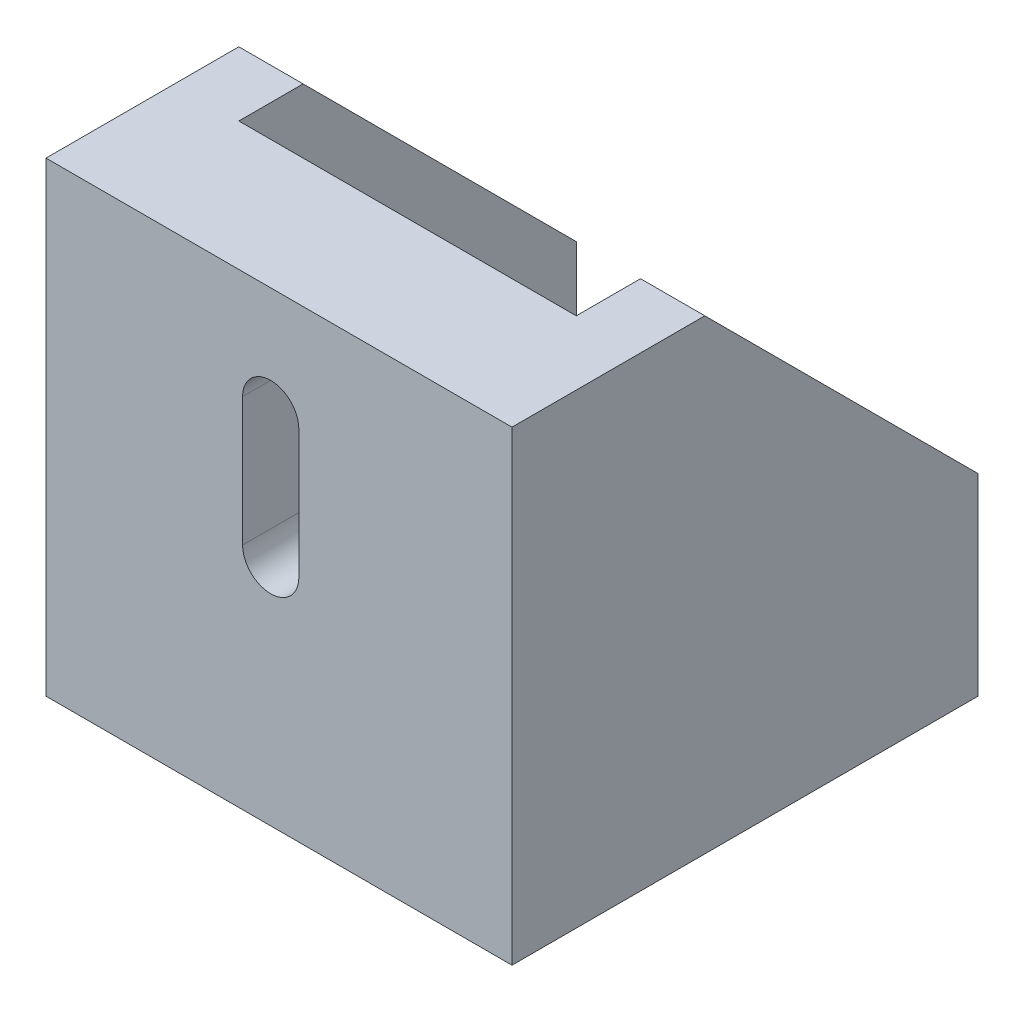
ISO-10303-21;
HEADER;
FILE_DESCRIPTION(('STEP AP214'),'2;1');
FILE_NAME('part.step','',(''),(''),'','','');
FILE_SCHEMA(('AUTOMOTIVE_DESIGN { 1 0 10303 214 1 1 1 1 }'));
ENDSEC;
DATA;
#1=APPLICATION_CONTEXT('core data for automotive mechanical design processes');
#2=APPLICATION_PROTOCOL_DEFINITION('international standard','automotive_design',2000,#1);
#3=PRODUCT_CONTEXT('',#1,'mechanical');
#4=PRODUCT('Part','Part','',(#3));
#5=PRODUCT_RELATED_PRODUCT_CATEGORY('part','',(#4));
#6=PRODUCT_DEFINITION_FORMATION('','',#4);
#7=PRODUCT_DEFINITION_CONTEXT('part definition',#1,'design');
#8=PRODUCT_DEFINITION('design','',#6,#7);
#9=PRODUCT_DEFINITION_SHAPE('','',#8);
#10=(LENGTH_UNIT() NAMED_UNIT(*) SI_UNIT(.MILLI.,.METRE.));
#11=(NAMED_UNIT(*) PLANE_ANGLE_UNIT() SI_UNIT($,.RADIAN.));
#12=(NAMED_UNIT(*) SI_UNIT($,.STERADIAN.) SOLID_ANGLE_UNIT());
#13=UNCERTAINTY_MEASURE_WITH_UNIT(LENGTH_MEASURE(1.E-05),#10,'distance_accuracy_value','');
#14=(GEOMETRIC_REPRESENTATION_CONTEXT(3) GLOBAL_UNCERTAINTY_ASSIGNED_CONTEXT((#13)) GLOBAL_UNIT_ASSIGNED_CONTEXT((#10,
#11,#12)) REPRESENTATION_CONTEXT('',''));
#15=CARTESIAN_POINT('',(0.,0.,0.));
#16=DIRECTION('',(0.,0.,1.));
#17=DIRECTION('',(1.,0.,0.));
#18=AXIS2_PLACEMENT_3D('',#15,#16,#17);
#19=CARTESIAN_POINT('',(0.,0.,0.));
#20=DIRECTION('',(0.,0.,1.));
#21=DIRECTION('',(1.,0.,0.));
#22=AXIS2_PLACEMENT_3D('',#19,#20,#21);
#23=PLANE('',#22);
#24=DIRECTION('',(0.,1.,0.));
#25=VECTOR('',#24,1.);
#26=CARTESIAN_POINT('',(15.7341445052597,14.2626530838324,0.));
#27=LINE('',#26,#25);
#28=CARTESIAN_POINT('',(15.7341445052597,14.2626530838324,0.));
#29=VERTEX_POINT('',#28);
#30=CARTESIAN_POINT('',(15.7341445052597,22.2626530838324,0.));
#31=VERTEX_POINT('',#30);
#32=EDGE_CURVE('E252',#29,#31,#27,.T.);
#33=ORIENTED_EDGE('',*,*,#32,.T.);
#34=CARTESIAN_POINT('',(13.9841445052597,22.2626530838324,0.));
#35=DIRECTION('',(0.,0.,1.));
#36=DIRECTION('',(1.,0.,0.));
#37=AXIS2_PLACEMENT_3D('',#34,#35,#36);
#38=CIRCLE('',#37,1.75);
#39=CARTESIAN_POINT('',(12.2341445052597,22.2626530838324,0.));
#40=VERTEX_POINT('',#39);
#41=EDGE_CURVE('E241',#31,#40,#38,.T.);
#42=ORIENTED_EDGE('',*,*,#41,.T.);
#43=DIRECTION('',(0.,-1.,0.));
#44=VECTOR('',#43,1.);
#45=CARTESIAN_POINT('',(12.2341445052597,22.2626530838324,0.));
#46=LINE('',#45,#44);
#47=CARTESIAN_POINT('',(12.2341445052597,14.2626530838324,0.));
#48=VERTEX_POINT('',#47);
#49=EDGE_CURVE('E242',#40,#48,#46,.T.);
#50=ORIENTED_EDGE('',*,*,#49,.T.);
#51=CARTESIAN_POINT('',(13.9841445052597,14.2626530838324,0.));
#52=DIRECTION('',(0.,0.,1.));
#53=DIRECTION('',(1.,0.,0.));
#54=AXIS2_PLACEMENT_3D('',#51,#52,#53);
#55=CIRCLE('',#54,1.75);
#56=EDGE_CURVE('E247',#48,#29,#55,.T.);
#57=ORIENTED_EDGE('',*,*,#56,.T.);
#58=EDGE_LOOP('',(#33,#42,#50,#57));
#59=FACE_BOUND('',#58,.T.);
#60=DIRECTION('',(-1.,0.,0.));
#61=VECTOR('',#60,1.);
#62=CARTESIAN_POINT('',(0.,8.,0.));
#63=LINE('',#62,#61);
#64=CARTESIAN_POINT('',(25.,8.,0.));
#65=VERTEX_POINT('',#64);
#66=CARTESIAN_POINT('',(4.,8.00000000000001,0.));
#67=VERTEX_POINT('',#66);
#68=EDGE_CURVE('E184',#65,#67,#63,.T.);
#69=ORIENTED_EDGE('',*,*,#68,.T.);
#70=DIRECTION('',(0.,1.,0.));
#71=VECTOR('',#70,1.);
#72=CARTESIAN_POINT('',(4.,29.,0.));
#73=LINE('',#72,#71);
#74=CARTESIAN_POINT('',(4.,29.,0.));
#75=VERTEX_POINT('',#74);
#76=EDGE_CURVE('E175',#67,#75,#73,.T.);
#77=ORIENTED_EDGE('',*,*,#76,.T.);
#78=DIRECTION('',(-1.,0.,0.));
#79=VECTOR('',#78,1.);
#80=CARTESIAN_POINT('',(29.,29.,0.));
#81=LINE('',#80,#79);
#82=CARTESIAN_POINT('',(25.,29.,0.));
#83=VERTEX_POINT('',#82);
#84=EDGE_CURVE('E182',#83,#75,#81,.T.);
#85=ORIENTED_EDGE('',*,*,#84,.F.);
#86=DIRECTION('',(0.,-1.,0.));
#87=VECTOR('',#86,1.);
#88=CARTESIAN_POINT('',(25.,29.,0.));
#89=LINE('',#88,#87);
#90=EDGE_CURVE('E282',#83,#65,#89,.T.);
#91=ORIENTED_EDGE('',*,*,#90,.T.);
#92=EDGE_LOOP('',(#69,#77,#85,#91));
#93=FACE_BOUND('',#92,.T.);
#94=ADVANCED_FACE('F44',(#59,#93),#23,.F.);
#95=CARTESIAN_POINT('',(0.,8.,0.));
#96=DIRECTION('',(0.,1.,0.));
#97=DIRECTION('',(0.,0.,1.));
#98=AXIS2_PLACEMENT_3D('',#95,#96,#97);
#99=PLANE('',#98);
#100=DIRECTION('',(0.,0.,1.));
#101=VECTOR('',#100,1.);
#102=CARTESIAN_POINT('',(4.,8.00000000000001,0.));
#103=LINE('',#102,#101);
#104=CARTESIAN_POINT('',(4.,8.,-21.));
#105=VERTEX_POINT('',#104);
#106=EDGE_CURVE('E58',#105,#67,#103,.T.);
#107=ORIENTED_EDGE('',*,*,#106,.T.);
#108=ORIENTED_EDGE('',*,*,#68,.F.);
#109=DIRECTION('',(0.,0.,-1.));
#110=VECTOR('',#109,1.);
#111=CARTESIAN_POINT('',(25.,8.,0.));
#112=LINE('',#111,#110);
#113=CARTESIAN_POINT('',(25.,8.,-21.));
#114=VERTEX_POINT('',#113);
#115=EDGE_CURVE('E293',#65,#114,#112,.T.);
#116=ORIENTED_EDGE('',*,*,#115,.T.);
#117=DIRECTION('',(1.,0.,0.));
#118=VECTOR('',#117,1.);
#119=CARTESIAN_POINT('',(29.,8.,-21.));
#120=LINE('',#119,#118);
#121=EDGE_CURVE('E234',#105,#114,#120,.T.);
#122=ORIENTED_EDGE('',*,*,#121,.F.);
#123=EDGE_LOOP('',(#107,#108,#116,#122));
#124=FACE_BOUND('',#123,.T.);
#125=CARTESIAN_POINT('',(13.9421842183201,8.,-15.));
#126=DIRECTION('',(0.,1.,0.));
#127=DIRECTION('',(0.,0.,1.));
#128=AXIS2_PLACEMENT_3D('',#125,#126,#127);
#129=CIRCLE('',#128,1.75);
#130=CARTESIAN_POINT('',(15.6921842183201,8.,-15.));
#131=VERTEX_POINT('',#130);
#132=CARTESIAN_POINT('',(12.1921842183201,8.,-15.));
#133=VERTEX_POINT('',#132);
#134=EDGE_CURVE('E303',#131,#133,#129,.T.);
#135=ORIENTED_EDGE('',*,*,#134,.F.);
#136=DIRECTION('',(0.,0.,-1.));
#137=VECTOR('',#136,1.);
#138=CARTESIAN_POINT('',(15.6921842183201,8.,-7.00000000000001));
#139=LINE('',#138,#137);
#140=CARTESIAN_POINT('',(15.6921842183201,8.,-7.00000000000001));
#141=VERTEX_POINT('',#140);
#142=EDGE_CURVE('E307',#141,#131,#139,.T.);
#143=ORIENTED_EDGE('',*,*,#142,.F.);
#144=CARTESIAN_POINT('',(13.9421842183201,8.,-7.00000000000001));
#145=DIRECTION('',(0.,1.,0.));
#146=DIRECTION('',(0.,0.,1.));
#147=AXIS2_PLACEMENT_3D('',#144,#145,#146);
#148=CIRCLE('',#147,1.75);
#149=CARTESIAN_POINT('',(12.1921842183201,8.,-7.00000000000001));
#150=VERTEX_POINT('',#149);
#151=EDGE_CURVE('E322',#150,#141,#148,.T.);
#152=ORIENTED_EDGE('',*,*,#151,.F.);
#153=DIRECTION('',(0.,0.,1.));
#154=VECTOR('',#153,1.);
#155=CARTESIAN_POINT('',(12.1921842183201,8.,-15.));
#156=LINE('',#155,#154);
#157=EDGE_CURVE('E319',#133,#150,#156,.T.);
#158=ORIENTED_EDGE('',*,*,#157,.F.);
#159=EDGE_LOOP('',(#135,#143,#152,#158));
#160=FACE_BOUND('',#159,.T.);
#161=ADVANCED_FACE('F339',(#124,#160),#99,.T.);
#162=CARTESIAN_POINT('',(0.,29.,8.));
#163=DIRECTION('',(1.,0.,0.));
#164=DIRECTION('',(0.,0.,-1.));
#165=AXIS2_PLACEMENT_3D('',#162,#163,#164);
#166=PLANE('',#165);
#167=DIRECTION('',(0.,0.,-1.));
#168=VECTOR('',#167,1.);
#169=CARTESIAN_POINT('',(0.,29.,8.));
#170=LINE('',#169,#168);
#171=CARTESIAN_POINT('',(0.,29.,8.));
#172=VERTEX_POINT('',#171);
#173=CARTESIAN_POINT('',(0.,29.,-4.));
#174=VERTEX_POINT('',#173);
#175=EDGE_CURVE('E201',#172,#174,#170,.T.);
#176=ORIENTED_EDGE('',*,*,#175,.T.);
#177=DIRECTION('',(0.,-0.707106781186547,-0.707106781186548));
#178=VECTOR('',#177,1.);
#179=CARTESIAN_POINT('',(0.,12.,-21.));
#180=LINE('',#179,#178);
#181=CARTESIAN_POINT('',(0.,12.,-21.));
#182=VERTEX_POINT('',#181);
#183=EDGE_CURVE('E187',#174,#182,#180,.T.);
#184=ORIENTED_EDGE('',*,*,#183,.T.);
#185=DIRECTION('',(0.,-1.,0.));
#186=VECTOR('',#185,1.);
#187=CARTESIAN_POINT('',(0.,8.,-21.));
#188=LINE('',#187,#186);
#189=CARTESIAN_POINT('',(0.,0.,-21.));
#190=VERTEX_POINT('',#189);
#191=EDGE_CURVE('E227',#182,#190,#188,.T.);
#192=ORIENTED_EDGE('',*,*,#191,.T.);
#193=DIRECTION('',(0.,0.,-1.));
#194=VECTOR('',#193,1.);
#195=CARTESIAN_POINT('',(0.,0.,8.));
#196=LINE('',#195,#194);
#197=CARTESIAN_POINT('',(0.,0.,8.));
#198=VERTEX_POINT('',#197);
#199=EDGE_CURVE('E11',#198,#190,#196,.T.);
#200=ORIENTED_EDGE('',*,*,#199,.F.);
#201=DIRECTION('',(0.,-1.,0.));
#202=VECTOR('',#201,1.);
#203=CARTESIAN_POINT('',(0.,29.,8.));
#204=LINE('',#203,#202);
#205=EDGE_CURVE('E195',#172,#198,#204,.T.);
#206=ORIENTED_EDGE('',*,*,#205,.F.);
#207=EDGE_LOOP('',(#176,#184,#192,#200,#206));
#208=FACE_BOUND('',#207,.T.);
#209=ADVANCED_FACE('F50',(#208),#166,.F.);
#210=CARTESIAN_POINT('',(0.,0.,8.));
#211=DIRECTION('',(0.,1.,0.));
#212=DIRECTION('',(0.,0.,1.));
#213=AXIS2_PLACEMENT_3D('',#210,#211,#212);
#214=PLANE('',#213);
#215=DIRECTION('',(0.,0.,-1.));
#216=VECTOR('',#215,1.);
#217=CARTESIAN_POINT('',(15.6921842183201,0.,-7.00000000000001));
#218=LINE('',#217,#216);
#219=CARTESIAN_POINT('',(15.6921842183201,0.,-7.00000000000001));
#220=VERTEX_POINT('',#219);
#221=CARTESIAN_POINT('',(15.6921842183201,0.,-15.));
#222=VERTEX_POINT('',#221);
#223=EDGE_CURVE('E312',#220,#222,#218,.T.);
#224=ORIENTED_EDGE('',*,*,#223,.T.);
#225=CARTESIAN_POINT('',(13.9421842183201,0.,-15.));
#226=DIRECTION('',(0.,1.,0.));
#227=DIRECTION('',(0.,0.,1.));
#228=AXIS2_PLACEMENT_3D('',#225,#226,#227);
#229=CIRCLE('',#228,1.75);
#230=CARTESIAN_POINT('',(12.1921842183201,0.,-15.));
#231=VERTEX_POINT('',#230);
#232=EDGE_CURVE('E304',#222,#231,#229,.T.);
#233=ORIENTED_EDGE('',*,*,#232,.T.);
#234=DIRECTION('',(0.,0.,1.));
#235=VECTOR('',#234,1.);
#236=CARTESIAN_POINT('',(12.1921842183201,0.,-15.));
#237=LINE('',#236,#235);
#238=CARTESIAN_POINT('',(12.1921842183201,0.,-7.00000000000001));
#239=VERTEX_POINT('',#238);
#240=EDGE_CURVE('E308',#231,#239,#237,.T.);
#241=ORIENTED_EDGE('',*,*,#240,.T.);
#242=CARTESIAN_POINT('',(13.9421842183201,0.,-7.00000000000001));
#243=DIRECTION('',(0.,1.,0.));
#244=DIRECTION('',(0.,0.,1.));
#245=AXIS2_PLACEMENT_3D('',#242,#243,#244);
#246=CIRCLE('',#245,1.75);
#247=EDGE_CURVE('E68',#239,#220,#246,.T.);
#248=ORIENTED_EDGE('',*,*,#247,.T.);
#249=EDGE_LOOP('',(#224,#233,#241,#248));
#250=FACE_BOUND('',#249,.T.);
#251=ORIENTED_EDGE('',*,*,#199,.T.);
#252=DIRECTION('',(1.,0.,0.));
#253=VECTOR('',#252,1.);
#254=CARTESIAN_POINT('',(29.,0.,-21.));
#255=LINE('',#254,#253);
#256=CARTESIAN_POINT('',(29.,0.,-21.));
#257=VERTEX_POINT('',#256);
#258=EDGE_CURVE('E224',#190,#257,#255,.T.);
#259=ORIENTED_EDGE('',*,*,#258,.T.);
#260=DIRECTION('',(0.,0.,-1.));
#261=VECTOR('',#260,1.);
#262=CARTESIAN_POINT('',(29.,0.,8.));
#263=LINE('',#262,#261);
#264=CARTESIAN_POINT('',(29.,0.,8.));
#265=VERTEX_POINT('',#264);
#266=EDGE_CURVE('E52',#265,#257,#263,.T.);
#267=ORIENTED_EDGE('',*,*,#266,.F.);
#268=DIRECTION('',(1.,0.,0.));
#269=VECTOR('',#268,1.);
#270=CARTESIAN_POINT('',(0.,0.,8.));
#271=LINE('',#270,#269);
#272=EDGE_CURVE('E196',#198,#265,#271,.T.);
#273=ORIENTED_EDGE('',*,*,#272,.F.);
#274=EDGE_LOOP('',(#251,#259,#267,#273));
#275=FACE_BOUND('',#274,.T.);
#276=ADVANCED_FACE('F230',(#250,#275),#214,.F.);
#277=CARTESIAN_POINT('',(29.,0.,8.));
#278=DIRECTION('',(-1.,0.,0.));
#279=DIRECTION('',(0.,0.,1.));
#280=AXIS2_PLACEMENT_3D('',#277,#278,#279);
#281=PLANE('',#280);
#282=DIRECTION('',(0.,0.707106781186547,0.707106781186547));
#283=VECTOR('',#282,1.);
#284=CARTESIAN_POINT('',(29.,29.,-4.));
#285=LINE('',#284,#283);
#286=CARTESIAN_POINT('',(29.,12.,-21.));
#287=VERTEX_POINT('',#286);
#288=CARTESIAN_POINT('',(29.,29.,-4.));
#289=VERTEX_POINT('',#288);
#290=EDGE_CURVE('E285',#287,#289,#285,.T.);
#291=ORIENTED_EDGE('',*,*,#290,.T.);
#292=DIRECTION('',(0.,0.,-1.));
#293=VECTOR('',#292,1.);
#294=CARTESIAN_POINT('',(29.,29.,8.));
#295=LINE('',#294,#293);
#296=CARTESIAN_POINT('',(29.,29.,8.));
#297=VERTEX_POINT('',#296);
#298=EDGE_CURVE('E207',#297,#289,#295,.T.);
#299=ORIENTED_EDGE('',*,*,#298,.F.);
#300=DIRECTION('',(0.,1.,0.));
#301=VECTOR('',#300,1.);
#302=CARTESIAN_POINT('',(29.,0.,8.));
#303=LINE('',#302,#301);
#304=EDGE_CURVE('E216',#265,#297,#303,.T.);
#305=ORIENTED_EDGE('',*,*,#304,.F.);
#306=ORIENTED_EDGE('',*,*,#266,.T.);
#307=DIRECTION('',(0.,-1.,0.));
#308=VECTOR('',#307,1.);
#309=CARTESIAN_POINT('',(29.,8.,-21.));
#310=LINE('',#309,#308);
#311=EDGE_CURVE('E214',#287,#257,#310,.T.);
#312=ORIENTED_EDGE('',*,*,#311,.F.);
#313=EDGE_LOOP('',(#291,#299,#305,#306,#312));
#314=FACE_BOUND('',#313,.T.);
#315=ADVANCED_FACE('F215',(#314),#281,.F.);
#316=CARTESIAN_POINT('',(29.,29.,8.));
#317=DIRECTION('',(0.,-1.,0.));
#318=DIRECTION('',(0.,0.,-1.));
#319=AXIS2_PLACEMENT_3D('',#316,#317,#318);
#320=PLANE('',#319);
#321=ORIENTED_EDGE('',*,*,#298,.T.);
#322=DIRECTION('',(1.,0.,0.));
#323=VECTOR('',#322,1.);
#324=CARTESIAN_POINT('',(25.,29.,-4.));
#325=LINE('',#324,#323);
#326=CARTESIAN_POINT('',(25.,29.,-4.));
#327=VERTEX_POINT('',#326);
#328=EDGE_CURVE('E297',#327,#289,#325,.T.);
#329=ORIENTED_EDGE('',*,*,#328,.F.);
#330=DIRECTION('',(0.,0.,1.));
#331=VECTOR('',#330,1.);
#332=CARTESIAN_POINT('',(25.,29.,0.));
#333=LINE('',#332,#331);
#334=EDGE_CURVE('E192',#327,#83,#333,.T.);
#335=ORIENTED_EDGE('',*,*,#334,.T.);
#336=ORIENTED_EDGE('',*,*,#84,.T.);
#337=DIRECTION('',(0.,0.,-1.));
#338=VECTOR('',#337,1.);
#339=CARTESIAN_POINT('',(4.,29.,0.));
#340=LINE('',#339,#338);
#341=CARTESIAN_POINT('',(4.,29.,-4.));
#342=VERTEX_POINT('',#341);
#343=EDGE_CURVE('E169',#75,#342,#340,.T.);
#344=ORIENTED_EDGE('',*,*,#343,.T.);
#345=DIRECTION('',(-1.,0.,0.));
#346=VECTOR('',#345,1.);
#347=CARTESIAN_POINT('',(4.,29.,-4.));
#348=LINE('',#347,#346);
#349=EDGE_CURVE('E274',#342,#174,#348,.T.);
#350=ORIENTED_EDGE('',*,*,#349,.T.);
#351=ORIENTED_EDGE('',*,*,#175,.F.);
#352=DIRECTION('',(-1.,0.,0.));
#353=VECTOR('',#352,1.);
#354=CARTESIAN_POINT('',(29.,29.,8.));
#355=LINE('',#354,#353);
#356=EDGE_CURVE('E204',#297,#172,#355,.T.);
#357=ORIENTED_EDGE('',*,*,#356,.F.);
#358=EDGE_LOOP('',(#321,#329,#335,#336,#344,#350,#351,#357));
#359=FACE_BOUND('',#358,.T.);
#360=ADVANCED_FACE('F186',(#359),#320,.F.);
#361=CARTESIAN_POINT('',(0.,0.,8.));
#362=DIRECTION('',(0.,0.,1.));
#363=DIRECTION('',(1.,0.,0.));
#364=AXIS2_PLACEMENT_3D('',#361,#362,#363);
#365=PLANE('',#364);
#366=CARTESIAN_POINT('',(13.9841445052597,22.2626530838324,8.));
#367=DIRECTION('',(0.,0.,1.));
#368=DIRECTION('',(1.,0.,0.));
#369=AXIS2_PLACEMENT_3D('',#366,#367,#368);
#370=CIRCLE('',#369,1.75);
#371=CARTESIAN_POINT('',(15.7341445052597,22.2626530838324,8.));
#372=VERTEX_POINT('',#371);
#373=CARTESIAN_POINT('',(12.2341445052597,22.2626530838324,8.));
#374=VERTEX_POINT('',#373);
#375=EDGE_CURVE('E228',#372,#374,#370,.T.);
#376=ORIENTED_EDGE('',*,*,#375,.F.);
#377=DIRECTION('',(0.,1.,0.));
#378=VECTOR('',#377,1.);
#379=CARTESIAN_POINT('',(15.7341445052597,14.2626530838324,8.));
#380=LINE('',#379,#378);
#381=CARTESIAN_POINT('',(15.7341445052597,14.2626530838324,8.));
#382=VERTEX_POINT('',#381);
#383=EDGE_CURVE('E244',#382,#372,#380,.T.);
#384=ORIENTED_EDGE('',*,*,#383,.F.);
#385=CARTESIAN_POINT('',(13.9841445052597,14.2626530838324,8.));
#386=DIRECTION('',(0.,0.,1.));
#387=DIRECTION('',(1.,0.,0.));
#388=AXIS2_PLACEMENT_3D('',#385,#386,#387);
#389=CIRCLE('',#388,1.75);
#390=CARTESIAN_POINT('',(12.2341445052597,14.2626530838324,8.));
#391=VERTEX_POINT('',#390);
#392=EDGE_CURVE('E256',#391,#382,#389,.T.);
#393=ORIENTED_EDGE('',*,*,#392,.F.);
#394=DIRECTION('',(0.,-1.,0.));
#395=VECTOR('',#394,1.);
#396=CARTESIAN_POINT('',(12.2341445052597,22.2626530838324,8.));
#397=LINE('',#396,#395);
#398=EDGE_CURVE('E257',#374,#391,#397,.T.);
#399=ORIENTED_EDGE('',*,*,#398,.F.);
#400=EDGE_LOOP('',(#376,#384,#393,#399));
#401=FACE_BOUND('',#400,.T.);
#402=ORIENTED_EDGE('',*,*,#205,.T.);
#403=ORIENTED_EDGE('',*,*,#272,.T.);
#404=ORIENTED_EDGE('',*,*,#304,.T.);
#405=ORIENTED_EDGE('',*,*,#356,.T.);
#406=EDGE_LOOP('',(#402,#403,#404,#405));
#407=FACE_BOUND('',#406,.T.);
#408=ADVANCED_FACE('F275',(#401,#407),#365,.T.);
#409=CARTESIAN_POINT('',(13.9841445052597,22.2626530838324,0.));
#410=DIRECTION('',(0.,0.,1.));
#411=DIRECTION('',(1.,0.,0.));
#412=AXIS2_PLACEMENT_3D('',#409,#410,#411);
#413=CYLINDRICAL_SURFACE('',#412,1.75);
#414=ORIENTED_EDGE('',*,*,#375,.T.);
#415=DIRECTION('',(0.,0.,1.));
#416=VECTOR('',#415,1.);
#417=CARTESIAN_POINT('',(12.2341445052597,22.2626530838324,0.));
#418=LINE('',#417,#416);
#419=EDGE_CURVE('E251',#40,#374,#418,.T.);
#420=ORIENTED_EDGE('',*,*,#419,.F.);
#421=ORIENTED_EDGE('',*,*,#41,.F.);
#422=DIRECTION('',(0.,0.,1.));
#423=VECTOR('',#422,1.);
#424=CARTESIAN_POINT('',(15.7341445052597,22.2626530838324,0.));
#425=LINE('',#424,#423);
#426=EDGE_CURVE('E194',#31,#372,#425,.T.);
#427=ORIENTED_EDGE('',*,*,#426,.T.);
#428=EDGE_LOOP('',(#414,#420,#421,#427));
#429=FACE_BOUND('',#428,.T.);
#430=ADVANCED_FACE('F491',(#429),#413,.F.);
#431=CARTESIAN_POINT('',(15.7341445052597,14.2626530838324,0.));
#432=DIRECTION('',(1.,0.,0.));
#433=DIRECTION('',(0.,0.,-1.));
#434=AXIS2_PLACEMENT_3D('',#431,#432,#433);
#435=PLANE('',#434);
#436=ORIENTED_EDGE('',*,*,#383,.T.);
#437=ORIENTED_EDGE('',*,*,#426,.F.);
#438=ORIENTED_EDGE('',*,*,#32,.F.);
#439=DIRECTION('',(0.,0.,1.));
#440=VECTOR('',#439,1.);
#441=CARTESIAN_POINT('',(15.7341445052597,14.2626530838324,0.));
#442=LINE('',#441,#440);
#443=EDGE_CURVE('E198',#29,#382,#442,.T.);
#444=ORIENTED_EDGE('',*,*,#443,.T.);
#445=EDGE_LOOP('',(#436,#437,#438,#444));
#446=FACE_BOUND('',#445,.T.);
#447=ADVANCED_FACE('F485',(#446),#435,.F.);
#448=CARTESIAN_POINT('',(13.9841445052597,14.2626530838324,0.));
#449=DIRECTION('',(0.,0.,1.));
#450=DIRECTION('',(1.,0.,0.));
#451=AXIS2_PLACEMENT_3D('',#448,#449,#450);
#452=CYLINDRICAL_SURFACE('',#451,1.75);
#453=ORIENTED_EDGE('',*,*,#392,.T.);
#454=ORIENTED_EDGE('',*,*,#443,.F.);
#455=ORIENTED_EDGE('',*,*,#56,.F.);
#456=DIRECTION('',(0.,0.,1.));
#457=VECTOR('',#456,1.);
#458=CARTESIAN_POINT('',(12.2341445052597,14.2626530838324,0.));
#459=LINE('',#458,#457);
#460=EDGE_CURVE('E264',#48,#391,#459,.T.);
#461=ORIENTED_EDGE('',*,*,#460,.T.);
#462=EDGE_LOOP('',(#453,#454,#455,#461));
#463=FACE_BOUND('',#462,.T.);
#464=ADVANCED_FACE('F471',(#463),#452,.F.);
#465=CARTESIAN_POINT('',(12.2341445052597,22.2626530838324,0.));
#466=DIRECTION('',(-1.,0.,0.));
#467=DIRECTION('',(0.,0.,1.));
#468=AXIS2_PLACEMENT_3D('',#465,#466,#467);
#469=PLANE('',#468);
#470=ORIENTED_EDGE('',*,*,#398,.T.);
#471=ORIENTED_EDGE('',*,*,#460,.F.);
#472=ORIENTED_EDGE('',*,*,#49,.F.);
#473=ORIENTED_EDGE('',*,*,#419,.T.);
#474=EDGE_LOOP('',(#470,#471,#472,#473));
#475=FACE_BOUND('',#474,.T.);
#476=ADVANCED_FACE('F392',(#475),#469,.F.);
#477=CARTESIAN_POINT('',(29.,8.,-21.));
#478=DIRECTION('',(0.,0.,-1.));
#479=DIRECTION('',(-1.,0.,0.));
#480=AXIS2_PLACEMENT_3D('',#477,#478,#479);
#481=PLANE('',#480);
#482=ORIENTED_EDGE('',*,*,#258,.F.);
#483=ORIENTED_EDGE('',*,*,#191,.F.);
#484=DIRECTION('',(-1.,0.,0.));
#485=VECTOR('',#484,1.);
#486=CARTESIAN_POINT('',(4.,12.,-21.));
#487=LINE('',#486,#485);
#488=CARTESIAN_POINT('',(4.,12.,-21.));
#489=VERTEX_POINT('',#488);
#490=EDGE_CURVE('E276',#489,#182,#487,.T.);
#491=ORIENTED_EDGE('',*,*,#490,.F.);
#492=DIRECTION('',(0.,-1.,0.));
#493=VECTOR('',#492,1.);
#494=CARTESIAN_POINT('',(4.,8.,-21.));
#495=LINE('',#494,#493);
#496=EDGE_CURVE('E589',#489,#105,#495,.T.);
#497=ORIENTED_EDGE('',*,*,#496,.T.);
#498=ORIENTED_EDGE('',*,*,#121,.T.);
#499=DIRECTION('',(0.,1.,0.));
#500=VECTOR('',#499,1.);
#501=CARTESIAN_POINT('',(25.,8.,-21.));
#502=LINE('',#501,#500);
#503=CARTESIAN_POINT('',(25.,12.,-21.));
#504=VERTEX_POINT('',#503);
#505=EDGE_CURVE('E295',#114,#504,#502,.T.);
#506=ORIENTED_EDGE('',*,*,#505,.T.);
#507=DIRECTION('',(1.,0.,0.));
#508=VECTOR('',#507,1.);
#509=CARTESIAN_POINT('',(25.,12.,-21.));
#510=LINE('',#509,#508);
#511=EDGE_CURVE('E221',#504,#287,#510,.T.);
#512=ORIENTED_EDGE('',*,*,#511,.T.);
#513=ORIENTED_EDGE('',*,*,#311,.T.);
#514=EDGE_LOOP('',(#482,#483,#491,#497,#498,#506,#512,#513));
#515=FACE_BOUND('',#514,.T.);
#516=ADVANCED_FACE('F222',(#515),#481,.T.);
#517=CARTESIAN_POINT('',(13.9421842183201,0.,-15.));
#518=DIRECTION('',(0.,1.,0.));
#519=DIRECTION('',(0.,0.,1.));
#520=AXIS2_PLACEMENT_3D('',#517,#518,#519);
#521=CYLINDRICAL_SURFACE('',#520,1.75);
#522=ORIENTED_EDGE('',*,*,#134,.T.);
#523=DIRECTION('',(0.,1.,0.));
#524=VECTOR('',#523,1.);
#525=CARTESIAN_POINT('',(12.1921842183201,0.,-15.));
#526=LINE('',#525,#524);
#527=EDGE_CURVE('E317',#231,#133,#526,.T.);
#528=ORIENTED_EDGE('',*,*,#527,.F.);
#529=ORIENTED_EDGE('',*,*,#232,.F.);
#530=DIRECTION('',(0.,1.,0.));
#531=VECTOR('',#530,1.);
#532=CARTESIAN_POINT('',(15.6921842183201,0.,-15.));
#533=LINE('',#532,#531);
#534=EDGE_CURVE('E235',#222,#131,#533,.T.);
#535=ORIENTED_EDGE('',*,*,#534,.T.);
#536=EDGE_LOOP('',(#522,#528,#529,#535));
#537=FACE_BOUND('',#536,.T.);
#538=ADVANCED_FACE('F341',(#537),#521,.F.);
#539=CARTESIAN_POINT('',(15.6921842183201,0.,-7.00000000000001));
#540=DIRECTION('',(1.,0.,0.));
#541=DIRECTION('',(0.,0.,-1.));
#542=AXIS2_PLACEMENT_3D('',#539,#540,#541);
#543=PLANE('',#542);
#544=ORIENTED_EDGE('',*,*,#142,.T.);
#545=ORIENTED_EDGE('',*,*,#534,.F.);
#546=ORIENTED_EDGE('',*,*,#223,.F.);
#547=DIRECTION('',(0.,1.,0.));
#548=VECTOR('',#547,1.);
#549=CARTESIAN_POINT('',(15.6921842183201,0.,-7.00000000000001));
#550=LINE('',#549,#548);
#551=EDGE_CURVE('E236',#220,#141,#550,.T.);
#552=ORIENTED_EDGE('',*,*,#551,.T.);
#553=EDGE_LOOP('',(#544,#545,#546,#552));
#554=FACE_BOUND('',#553,.T.);
#555=ADVANCED_FACE('F346',(#554),#543,.F.);
#556=CARTESIAN_POINT('',(13.9421842183201,0.,-7.00000000000001));
#557=DIRECTION('',(0.,1.,0.));
#558=DIRECTION('',(0.,0.,1.));
#559=AXIS2_PLACEMENT_3D('',#556,#557,#558);
#560=CYLINDRICAL_SURFACE('',#559,1.75);
#561=ORIENTED_EDGE('',*,*,#151,.T.);
#562=ORIENTED_EDGE('',*,*,#551,.F.);
#563=ORIENTED_EDGE('',*,*,#247,.F.);
#564=DIRECTION('',(0.,1.,0.));
#565=VECTOR('',#564,1.);
#566=CARTESIAN_POINT('',(12.1921842183201,0.,-7.00000000000001));
#567=LINE('',#566,#565);
#568=EDGE_CURVE('E330',#239,#150,#567,.T.);
#569=ORIENTED_EDGE('',*,*,#568,.T.);
#570=EDGE_LOOP('',(#561,#562,#563,#569));
#571=FACE_BOUND('',#570,.T.);
#572=ADVANCED_FACE('F342',(#571),#560,.F.);
#573=CARTESIAN_POINT('',(12.1921842183201,0.,-15.));
#574=DIRECTION('',(-1.,0.,0.));
#575=DIRECTION('',(0.,0.,1.));
#576=AXIS2_PLACEMENT_3D('',#573,#574,#575);
#577=PLANE('',#576);
#578=ORIENTED_EDGE('',*,*,#157,.T.);
#579=ORIENTED_EDGE('',*,*,#568,.F.);
#580=ORIENTED_EDGE('',*,*,#240,.F.);
#581=ORIENTED_EDGE('',*,*,#527,.T.);
#582=EDGE_LOOP('',(#578,#579,#580,#581));
#583=FACE_BOUND('',#582,.T.);
#584=ADVANCED_FACE('F335',(#583),#577,.F.);
#585=CARTESIAN_POINT('',(25.,29.,-4.));
#586=DIRECTION('',(0.,0.707106781186547,-0.707106781186547));
#587=DIRECTION('',(0.,0.707106781186548,0.707106781186548));
#588=AXIS2_PLACEMENT_3D('',#585,#586,#587);
#589=PLANE('',#588);
#590=ORIENTED_EDGE('',*,*,#290,.F.);
#591=ORIENTED_EDGE('',*,*,#511,.F.);
#592=DIRECTION('',(0.,0.707106781186547,0.707106781186547));
#593=VECTOR('',#592,1.);
#594=CARTESIAN_POINT('',(25.,29.,-4.));
#595=LINE('',#594,#593);
#596=EDGE_CURVE('E298',#504,#327,#595,.T.);
#597=ORIENTED_EDGE('',*,*,#596,.T.);
#598=ORIENTED_EDGE('',*,*,#328,.T.);
#599=EDGE_LOOP('',(#590,#591,#597,#598));
#600=FACE_BOUND('',#599,.T.);
#601=ADVANCED_FACE('F420',(#600),#589,.T.);
#602=CARTESIAN_POINT('',(25.,0.,0.));
#603=DIRECTION('',(1.,0.,0.));
#604=DIRECTION('',(0.,0.,-1.));
#605=AXIS2_PLACEMENT_3D('',#602,#603,#604);
#606=PLANE('',#605);
#607=ORIENTED_EDGE('',*,*,#90,.F.);
#608=ORIENTED_EDGE('',*,*,#334,.F.);
#609=ORIENTED_EDGE('',*,*,#596,.F.);
#610=ORIENTED_EDGE('',*,*,#505,.F.);
#611=ORIENTED_EDGE('',*,*,#115,.F.);
#612=EDGE_LOOP('',(#607,#608,#609,#610,#611));
#613=FACE_BOUND('',#612,.T.);
#614=ADVANCED_FACE('F405',(#613),#606,.F.);
#615=CARTESIAN_POINT('',(4.,12.,-21.));
#616=DIRECTION('',(0.,0.707106781186548,-0.707106781186547));
#617=DIRECTION('',(0.,0.707106781186547,0.707106781186548));
#618=AXIS2_PLACEMENT_3D('',#615,#616,#617);
#619=PLANE('',#618);
#620=ORIENTED_EDGE('',*,*,#183,.F.);
#621=ORIENTED_EDGE('',*,*,#349,.F.);
#622=DIRECTION('',(0.,-0.707106781186547,-0.707106781186548));
#623=VECTOR('',#622,1.);
#624=CARTESIAN_POINT('',(4.,12.,-21.));
#625=LINE('',#624,#623);
#626=EDGE_CURVE('E172',#342,#489,#625,.T.);
#627=ORIENTED_EDGE('',*,*,#626,.T.);
#628=ORIENTED_EDGE('',*,*,#490,.T.);
#629=EDGE_LOOP('',(#620,#621,#627,#628));
#630=FACE_BOUND('',#629,.T.);
#631=ADVANCED_FACE('F281',(#630),#619,.T.);
#632=CARTESIAN_POINT('',(4.,0.,0.));
#633=DIRECTION('',(1.,0.,0.));
#634=DIRECTION('',(0.,0.,-1.));
#635=AXIS2_PLACEMENT_3D('',#632,#633,#634);
#636=PLANE('',#635);
#637=ORIENTED_EDGE('',*,*,#76,.F.);
#638=ORIENTED_EDGE('',*,*,#106,.F.);
#639=ORIENTED_EDGE('',*,*,#496,.F.);
#640=ORIENTED_EDGE('',*,*,#626,.F.);
#641=ORIENTED_EDGE('',*,*,#343,.F.);
#642=EDGE_LOOP('',(#637,#638,#639,#640,#641));
#643=FACE_BOUND('',#642,.T.);
#644=ADVANCED_FACE('F171',(#643),#636,.T.);
#645=CLOSED_SHELL('',(#94,#161,#209,#276,#315,#360,#408,#430,#447,#464,#476,#516,#538,#555,#572,
#584,#601,#614,#631,#644));
#646=MANIFOLD_SOLID_BREP('B2',#645);
#647=ADVANCED_BREP_SHAPE_REPRESENTATION('',(#18,#646),#14);
#648=SHAPE_DEFINITION_REPRESENTATION(#9,#647);
ENDSEC;
END-ISO-10303-21;
